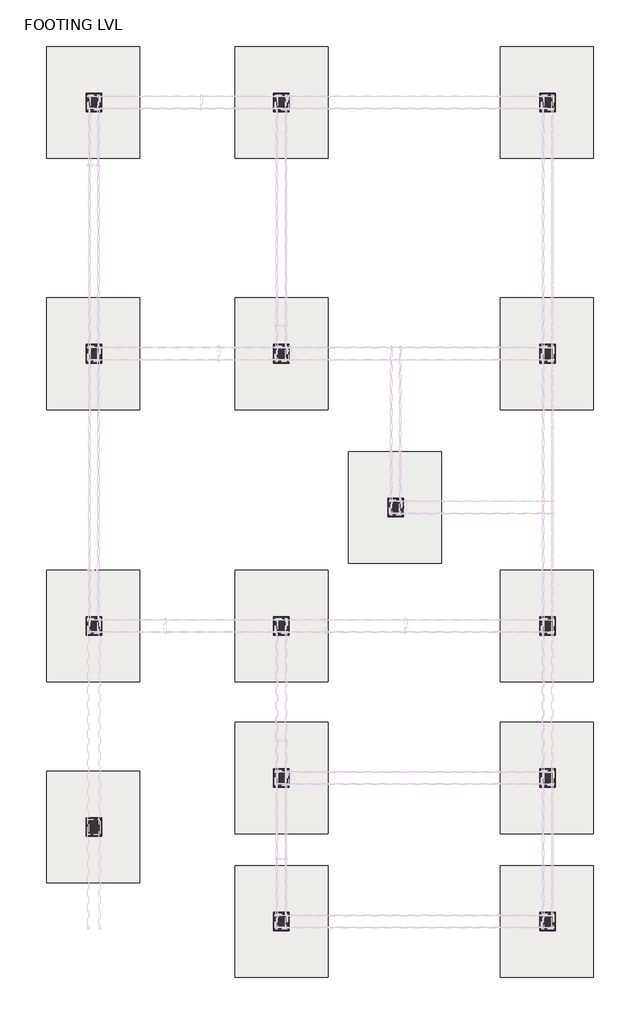
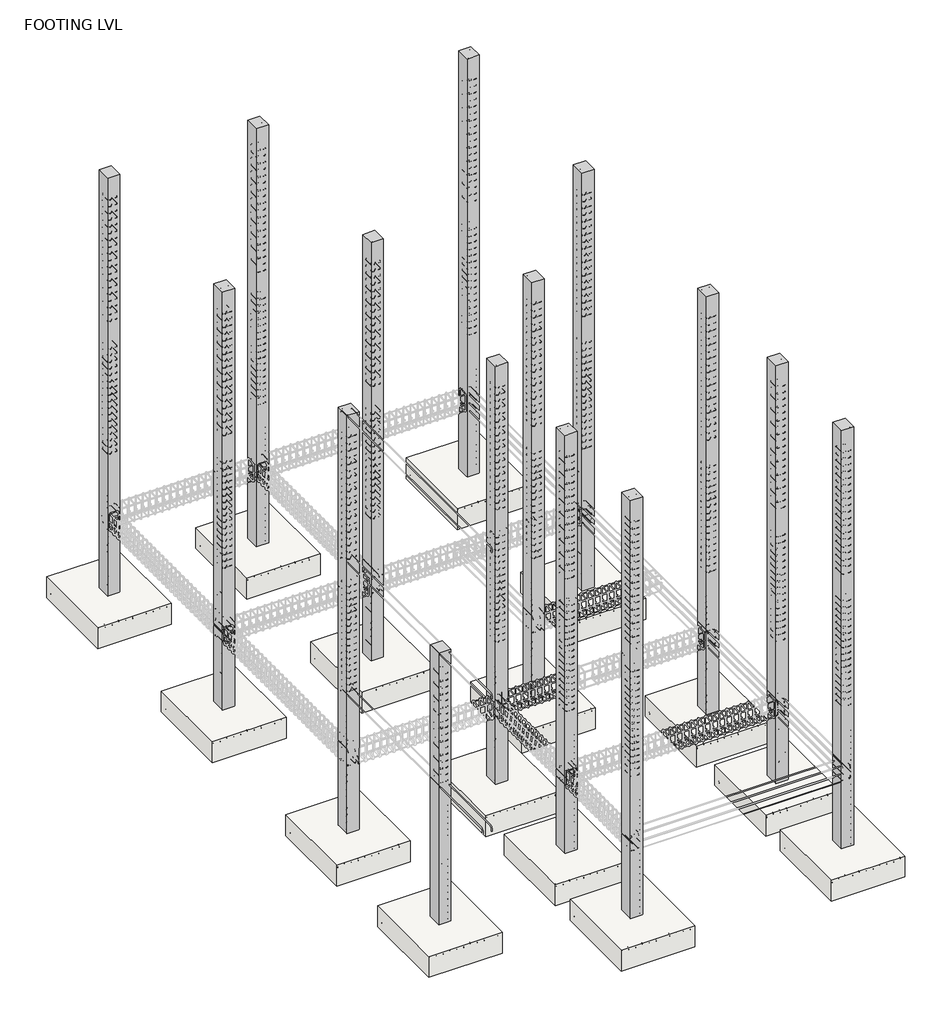
# One storey, part 1 of 16: 15 columns, 15 slabs.
"""IFC4 building model written with IfcOpenShell, lengths in millimetres."""

from ifc_helpers import new_model, si_unit, frame, origin, place, context, project, spatial, polyline, outline, extrude, transform, mapped, element, save
from components import footing_rectangular_5_x_6_26a6a031

model = new_model("IFC4")

# Units and contexts
model_context = context("Model", 3, world=origin())
ifc_project = project(units=[si_unit("LENGTHUNIT", "METRE", prefix="MILLI")], contexts=[model_context])

# Site, building, storey
site = spatial("IfcSite", under=ifc_project)
building = spatial("IfcBuilding", under=site)
storey = spatial("IfcBuildingStorey", under=building, Name="FOOTING LVL", Elevation=-1828.8)

# Columns
placement = place(None, origin())
element("IfcColumn", 1, ObjectType="Concrete-Rectangular-Column : 12 X10", at=placement, inside=storey, context=model_context, shape_type="SweptSolid", body=[
    extrude(outline(polyline([(-12555.8727572, 6368.8810259), (-12555.8727572, 6064.0810259), (-12809.8727572, 6064.0810259), (-12809.8727572, 6368.8810259), (-12555.8727572, 6368.8810259)])), frame((0.0, 0.0, -1828.8), z_axis=(0.0, 0.0, 1.0), x_axis=(1.0, 0.0, 0.0)), (0.0, 0.0, 1.0), 9144.0),
])
element("IfcColumn", 2, ObjectType="Concrete-Rectangular-Column : 12 X10", at=placement, inside=storey, context=model_context, shape_type="SweptSolid", body=[
    extrude(outline(polyline([(-9482.4727572, 6368.8810259), (-9482.4727572, 6064.0810259), (-9736.4727572, 6064.0810259), (-9736.4727572, 6368.8810259), (-9482.4727572, 6368.8810259)])), frame((0.0, 0.0, -1828.8), z_axis=(0.0, 0.0, 1.0), x_axis=(1.0, 0.0, 0.0)), (0.0, 0.0, 1.0), 9144.0),
])
element("IfcColumn", 3, ObjectType="Concrete-Rectangular-Column : 12 X10", at=placement, inside=storey, context=model_context, shape_type="SweptSolid", body=[
    extrude(outline(polyline([(-5119.2788618, 6368.8810259), (-5119.2788618, 6064.0810259), (-5373.2788618, 6064.0810259), (-5373.2788618, 6368.8810259), (-5119.2788618, 6368.8810259)])), frame((0.0, 0.0, -1828.8), z_axis=(0.0, 0.0, 1.0), x_axis=(1.0, 0.0, 0.0)), (0.0, 0.0, 1.0), 9144.0),
])
element("IfcColumn", 4, ObjectType="Concrete-Rectangular-Column : 12 X10", at=placement, inside=storey, context=model_context, shape_type="SweptSolid", body=[
    extrude(outline(polyline([(-5119.2788618, 10824.1780219), (-5119.2788618, 10519.3780219), (-5373.2788618, 10519.3780219), (-5373.2788618, 10824.1780219), (-5119.2788618, 10824.1780219)])), frame((0.0, 0.0, -1828.8), z_axis=(0.0, 0.0, 1.0), x_axis=(1.0, 0.0, 0.0)), (0.0, 0.0, 1.0), 9144.0),
])
element("IfcColumn", 5, ObjectType="Concrete-Rectangular-Column : 12 X10", at=placement, inside=storey, context=model_context, shape_type="SweptSolid", body=[
    extrude(outline(polyline([(-9482.4727572, 10824.1780219), (-9482.4727572, 10519.3780219), (-9736.4727572, 10519.3780219), (-9736.4727572, 10824.1780219), (-9482.4727572, 10824.1780219)])), frame((0.0, 0.0, -1828.8), z_axis=(0.0, 0.0, 1.0), x_axis=(1.0, 0.0, 0.0)), (0.0, 0.0, 1.0), 9144.0),
])
element("IfcColumn", 6, ObjectType="Concrete-Rectangular-Column : 12 X10", at=placement, inside=storey, context=model_context, shape_type="SweptSolid", body=[
    extrude(outline(polyline([(-12555.8727572, 10824.1780219), (-12555.8727572, 10519.3780219), (-12809.8727572, 10519.3780219), (-12809.8727572, 10824.1780219), (-12555.8727572, 10824.1780219)])), frame((0.0, 0.0, -1828.8), z_axis=(0.0, 0.0, 1.0), x_axis=(1.0, 0.0, 0.0)), (0.0, 0.0, 1.0), 9144.0),
])
element("IfcColumn", 7, ObjectType="Concrete-Rectangular-Column : 12 X10", at=placement, inside=storey, context=model_context, shape_type="SweptSolid", body=[
    extrude(outline(polyline([(-12555.8727572, 14938.9780219), (-12555.8727572, 14634.1780219), (-12809.8727572, 14634.1780219), (-12809.8727572, 14938.9780219), (-12555.8727572, 14938.9780219)])), frame((0.0, 0.0, -1828.8), z_axis=(0.0, 0.0, 1.0), x_axis=(1.0, 0.0, 0.0)), (0.0, 0.0, 1.0), 9144.0),
])
element("IfcColumn", 8, ObjectType="Concrete-Rectangular-Column : 12 X10", at=placement, inside=storey, context=model_context, shape_type="SweptSolid", body=[
    extrude(outline(polyline([(-9736.4727572, 14634.1780219), (-9736.4727572, 14938.9780219), (-9482.4727572, 14938.9780219), (-9482.4727572, 14634.1780219), (-9736.4727572, 14634.1780219)])), frame((0.0, 0.0, -1828.8), z_axis=(0.0, 0.0, 1.0), x_axis=(1.0, 0.0, 0.0)), (0.0, 0.0, 1.0), 9144.0),
])
element("IfcColumn", 9, ObjectType="Concrete-Rectangular-Column : 12 X10", at=placement, inside=storey, context=model_context, shape_type="SweptSolid", body=[
    extrude(outline(polyline([(-5373.2788618, 14634.1780219), (-5373.2788618, 14938.9780219), (-5119.2788618, 14938.9780219), (-5119.2788618, 14634.1780219), (-5373.2788618, 14634.1780219)])), frame((0.0, 0.0, -1828.8), z_axis=(0.0, 0.0, 1.0), x_axis=(1.0, 0.0, 0.0)), (0.0, 0.0, 1.0), 9144.0),
])
element("IfcColumn", 10, ObjectType="Concrete-Rectangular-Column : 12 X10", at=placement, inside=storey, context=model_context, shape_type="SweptSolid", body=[
    extrude(outline(polyline([(-5373.2788618, 3574.8810259), (-5373.2788618, 3879.6810259), (-5119.2788618, 3879.6810259), (-5119.2788618, 3574.8810259), (-5373.2788618, 3574.8810259)])), frame((0.0, 0.0, -1828.8), z_axis=(0.0, 0.0, 1.0), x_axis=(1.0, 0.0, 0.0)), (0.0, 0.0, 1.0), 9144.0),
])
element("IfcColumn", 11, ObjectType="Concrete-Rectangular-Column : 12 X10", at=placement, inside=storey, context=model_context, shape_type="SweptSolid", body=[
    extrude(outline(polyline([(-5373.2788618, 1223.5813769), (-5373.2788618, 1528.3813769), (-5119.2788618, 1528.3813769), (-5119.2788618, 1223.5813769), (-5373.2788618, 1223.5813769)])), frame((0.0, 0.0, -1828.8), z_axis=(0.0, 0.0, 1.0), x_axis=(1.0, 0.0, 0.0)), (0.0, 0.0, 1.0), 9144.0),
])
element("IfcColumn", 12, ObjectType="Concrete-Rectangular-Column : 12 X10", at=placement, inside=storey, context=model_context, shape_type="SweptSolid", body=[
    extrude(outline(polyline([(-9736.4727572, 1223.5813769), (-9736.4727572, 1528.3813769), (-9482.4727572, 1528.3813769), (-9482.4727572, 1223.5813769), (-9736.4727572, 1223.5813769)])), frame((0.0, 0.0, -1828.8), z_axis=(0.0, 0.0, 1.0), x_axis=(1.0, 0.0, 0.0)), (0.0, 0.0, 1.0), 9144.0),
])
element("IfcColumn", 13, ObjectType="Concrete-Rectangular-Column : 12 X10", at=placement, inside=storey, context=model_context, shape_type="SweptSolid", body=[
    extrude(outline(polyline([(-9736.4727572, 3574.8810259), (-9736.4727572, 3879.6810259), (-9482.4727572, 3879.6810259), (-9482.4727572, 3574.8810259), (-9736.4727572, 3574.8810259)])), frame((0.0, 0.0, -1828.8), z_axis=(0.0, 0.0, 1.0), x_axis=(1.0, 0.0, 0.0)), (0.0, 0.0, 1.0), 9144.0),
])
element("IfcColumn", 14, ObjectType="Concrete-Rectangular-Column : 12 X10", at=placement, inside=storey, context=model_context, shape_type="SweptSolid", body=[
    extrude(outline(polyline([(-12809.8727572, 2772.9813769), (-12809.8727572, 3077.7813769), (-12555.8727572, 3077.7813769), (-12555.8727572, 2772.9813769), (-12809.8727572, 2772.9813769)])), frame((0.0, 0.0, -1828.8), z_axis=(0.0, 0.0, 1.0), x_axis=(1.0, 0.0, 0.0)), (0.0, 0.0, 1.0), 5943.6),
])
element("IfcColumn", 15, ObjectType="Concrete-Rectangular-Column : 12 X10", at=placement, inside=storey, context=model_context, shape_type="SweptSolid", body=[
    extrude(outline(polyline([(-7608.4788618, 8309.5780219), (-7608.4788618, 8004.7780219), (-7862.4788618, 8004.7780219), (-7862.4788618, 8309.5780219), (-7608.4788618, 8309.5780219)])), frame((0.0, 0.0, -1828.8), z_axis=(0.0, 0.0, 1.0), x_axis=(1.0, 0.0, 0.0)), (0.0, 0.0, 1.0), 9144.0),
])

# Slabs
footing_rectangular_5_x_6_shape = footing_rectangular_5_x_6_26a6a031(model_context)
element("IfcSlab", 16, ObjectType="Footing-Rectangular : 5' X 6", at=placement, inside=storey, context=model_context, shape_type="MappedRepresentation", body=[
    mapped(footing_rectangular_5_x_6_shape, transform((-12696.3321567, 14786.5780219, -1828.8), x_axis=(1.0, 0.0, 0.0), y_axis=(0.0, 1.0, 0.0), z_axis=(0.0, 0.0, 1.0))),
])
element("IfcSlab", 17, ObjectType="Footing-Rectangular : 5' X 6", at=placement, inside=storey, context=model_context, shape_type="MappedRepresentation", body=[
    mapped(footing_rectangular_5_x_6_shape, transform((-9609.4727572, 14786.5780219, -1828.8), x_axis=(-1.0, 0.0, 0.0), y_axis=(0.0, -1.0, 0.0), z_axis=(0.0, 0.0, 1.0))),
])
element("IfcSlab", 18, ObjectType="Footing-Rectangular : 5' X 6", at=placement, inside=storey, context=model_context, shape_type="MappedRepresentation", body=[
    mapped(footing_rectangular_5_x_6_shape, transform((-5259.7382613, 14786.5780219, -1828.8), x_axis=(-1.0, 0.0, 0.0), y_axis=(0.0, -1.0, 0.0), z_axis=(0.0, 0.0, 1.0))),
])
element("IfcSlab", 19, ObjectType="Footing-Rectangular : 5' X 6", at=placement, inside=storey, context=model_context, shape_type="MappedRepresentation", body=[
    mapped(footing_rectangular_5_x_6_shape, transform((-5259.7382613, 10671.7780219, -1828.8), x_axis=(-1.0, 0.0, 0.0), y_axis=(0.0, -1.0, 0.0), z_axis=(0.0, 0.0, 1.0))),
])
element("IfcSlab", 20, ObjectType="Footing-Rectangular : 5' X 6", at=placement, inside=storey, context=model_context, shape_type="MappedRepresentation", body=[
    mapped(footing_rectangular_5_x_6_shape, transform((-9609.4727572, 10671.7780219, -1828.8), x_axis=(-1.0, 0.0, 0.0), y_axis=(0.0, -1.0, 0.0), z_axis=(0.0, 0.0, 1.0))),
])
element("IfcSlab", 21, ObjectType="Footing-Rectangular : 5' X 6", at=placement, inside=storey, context=model_context, shape_type="MappedRepresentation", body=[
    mapped(footing_rectangular_5_x_6_shape, transform((-12696.3321567, 10671.7780219, -1828.8), x_axis=(-1.0, 0.0, 0.0), y_axis=(0.0, -1.0, 0.0), z_axis=(0.0, 0.0, 1.0))),
])
element("IfcSlab", 22, ObjectType="Footing-Rectangular : 5' X 6", at=placement, inside=storey, context=model_context, shape_type="MappedRepresentation", body=[
    mapped(footing_rectangular_5_x_6_shape, transform((-7748.9382613, 8157.1780219, -1828.8), x_axis=(-1.0, 0.0, 0.0), y_axis=(0.0, -1.0, 0.0), z_axis=(0.0, 0.0, 1.0))),
])
element("IfcSlab", 23, ObjectType="Footing-Rectangular : 5' X 6", at=placement, inside=storey, context=model_context, shape_type="MappedRepresentation", body=[
    mapped(footing_rectangular_5_x_6_shape, transform((-9609.4727572, 6216.4810259, -1828.8), x_axis=(-1.0, 0.0, 0.0), y_axis=(0.0, -1.0, 0.0), z_axis=(0.0, 0.0, 1.0))),
])
element("IfcSlab", 24, ObjectType="Footing-Rectangular : 5' X 6", at=placement, inside=storey, context=model_context, shape_type="MappedRepresentation", body=[
    mapped(footing_rectangular_5_x_6_shape, transform((-5259.7382613, 6216.4810259, -1828.8), x_axis=(-1.0, 0.0, 0.0), y_axis=(0.0, -1.0, 0.0), z_axis=(0.0, 0.0, 1.0))),
])
element("IfcSlab", 25, ObjectType="Footing-Rectangular : 5' X 6", at=placement, inside=storey, context=model_context, shape_type="MappedRepresentation", body=[
    mapped(footing_rectangular_5_x_6_shape, transform((-5259.7382613, 3727.2810259, -1828.8), x_axis=(-1.0, 0.0, 0.0), y_axis=(0.0, -1.0, 0.0), z_axis=(0.0, 0.0, 1.0))),
])
element("IfcSlab", 26, ObjectType="Footing-Rectangular : 5' X 6", at=placement, inside=storey, context=model_context, shape_type="MappedRepresentation", body=[
    mapped(footing_rectangular_5_x_6_shape, transform((-9609.4727572, 3727.2810259, -1828.8), x_axis=(-1.0, 0.0, 0.0), y_axis=(0.0, -1.0, 0.0), z_axis=(0.0, 0.0, 1.0))),
])
element("IfcSlab", 27, ObjectType="Footing-Rectangular : 5' X 6", at=placement, inside=storey, context=model_context, shape_type="MappedRepresentation", body=[
    mapped(footing_rectangular_5_x_6_shape, transform((-12696.3321567, 6216.4810259, -1828.8), x_axis=(-1.0, 0.0, 0.0), y_axis=(0.0, -1.0, 0.0), z_axis=(0.0, 0.0, 1.0))),
])
element("IfcSlab", 28, ObjectType="Footing-Rectangular : 5' X 6", at=placement, inside=storey, context=model_context, shape_type="MappedRepresentation", body=[
    mapped(footing_rectangular_5_x_6_shape, transform((-12696.3321567, 2925.3813769, -1828.8), x_axis=(-1.0, 0.0, 0.0), y_axis=(0.0, -1.0, 0.0), z_axis=(0.0, 0.0, 1.0))),
])
element("IfcSlab", 29, ObjectType="Footing-Rectangular : 5' X 6", at=placement, inside=storey, context=model_context, shape_type="MappedRepresentation", body=[
    mapped(footing_rectangular_5_x_6_shape, transform((-9609.4727572, 1375.9813769, -1828.8), x_axis=(-1.0, 0.0, 0.0), y_axis=(0.0, -1.0, 0.0), z_axis=(0.0, 0.0, 1.0))),
])
element("IfcSlab", 30, ObjectType="Footing-Rectangular : 5' X 6", at=placement, inside=storey, context=model_context, shape_type="MappedRepresentation", body=[
    mapped(footing_rectangular_5_x_6_shape, transform((-5259.7382613, 1375.9813769, -1828.8), x_axis=(-1.0, 0.0, 0.0), y_axis=(0.0, -1.0, 0.0), z_axis=(0.0, 0.0, 1.0))),
])

save(model, "model.ifc")

# Revit data of these elements
# Grids (mm)
#   "1": line (422.406, 14786.578) -> (-17190.593, 14786.578)
#   "2": line (422.406, 10671.778) -> (-17190.593, 10671.778)
#   "3": line (422.406, 8157.178) -> (-17190.593, 8157.178)
#   "4": line (422.406, 6216.481) -> (-17190.593, 6216.481)
#   "5": line (422.406, 3727.281) -> (-17190.593, 3727.281)
#   "6": line (422.406, 2925.381) -> (-17190.593, 2925.381)
#   "7": line (422.406, 1375.981) -> (-17190.593, 1375.981)
#   "A": line (-12682.873, -3267.355) -> (-12682.873, 19328.969)
#   "C": line (-7735.479, -3267.355) -> (-7735.479, 19328.969)
#   "D": line (-5259.738, -3267.355) -> (-5259.738, 19328.969)
#   "B": line (-9609.473, -3267.355) -> (-9609.473, 19328.969)
# Type "Concrete-Rectangular-Column : 12 X10"
#   Assembly Code = "B10"
#   b = 0' - 10"
#   h = 1' - 0"
#   Structural Material [instance default] = Concrete, Cast-in-Place gray
# Type "Footing-Rectangular : 5' X 6"
#   Assembly Code = "A1010100"
#   Width = 5' - 0"
#   Length = 6' - 0"
#   Foundation Thickness = 1' - 6"
#   Structural Material [instance default] = Concrete, Cast-in-Place gray
# Elements 1, 2, 3, 4, 5, 6, 7, 8, 9, 10, 11, 12, 13, 14, 15 (IfcColumn, "Concrete-Rectangular-Column : 12 X10")
#   Structural Material = Concrete, Cast-in-Place gray
#   Phase Created = New Construction
#   Materials on its faces: "Concrete, Cast-in-Place gray"
# Elements 16, 17, 18, 19, 20, 21, 22, 23, 24, 25, 26, 27, 28, 29, 30 (IfcSlab, "Footing-Rectangular : 5' X 6")
#   Structural Material = Concrete, Cast-in-Place gray
#   Phase Created = New Construction
#   Materials on its faces: "Concrete, Cast-in-Place gray"
# Materials
#   "Concrete, Cast-in-Place gray": class "Concrete", colour RGB 192 192 192, transparency 0, Description = "Cast-in-place concrete", Cost = 0
